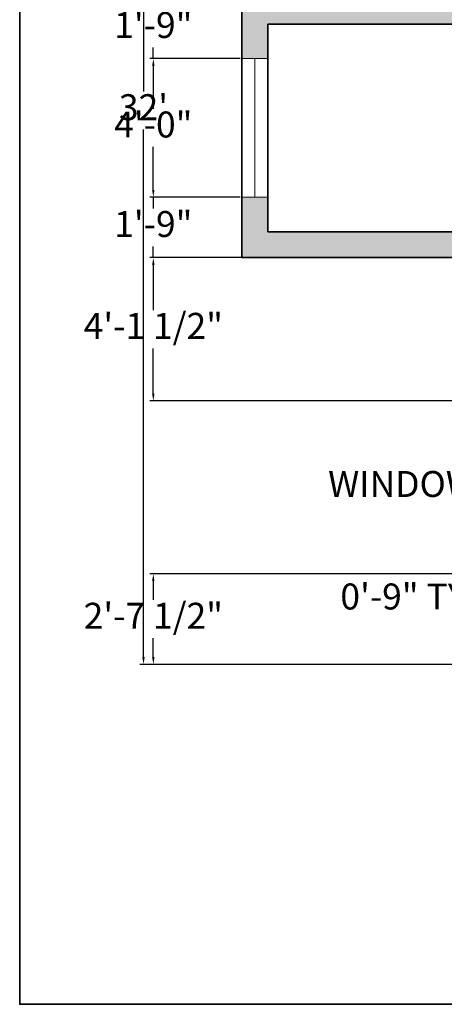
# Model space of a CAD drawing. Units: inches. Extents: x 1329 to 1989, y 1493 to 2072.
# Tile 1 of 4: x 1329 to 1476, y 1501 to 1842. Entities that reach past the tile are written whole.
import ezdxf

# ---------------------------------------------------------------- set-up
doc = ezdxf.new("R2010")
doc.units = ezdxf.units.IN
for name, color, linetype, lineweight in [('A-ANNO-DIMS', 2, 'Continuous', 18), ('A-ANNO-TTLB', 7, 'Continuous', 35), ('A-GLAZ', 4, 'Continuous', 18), ('A-WALL', 7, 'Continuous', 35)]:
    doc.layers.add(name, color=color, linetype=linetype, lineweight=lineweight)
doc.layers.add('A-WALL-PATT', color=251, linetype='Continuous', lineweight=13, true_color=0x636466)
doc.styles.get("Standard").update_dxf_attribs({"font": 'arial.ttf'})
doc.dimstyles.new('ISO-25', dxfattribs={"dimtxt": 9, "dimasz": 2.5, "dimexe": 1.25, "dimexo": 0.625, "dimgap": 2, "dimtad": 0, "dimtih": 1, "dimtoh": 1, "dimdec": 1, "dimlunit": 4, "dimtxsty": 'Standard', "dimcen": 2.5, "dimadec": 0, "dimazin": 0, "dimtfac": 0.5, "dimtdec": 1, "dimtmove": 0, "dimatfit": 3, "dimfxl": 1, "dimarcsym": 0})

# ---------------------------------------------------------------- blocks, each defined once
blk = doc.blocks.new('*D14')
at = {"layer": 'A-ANNO-DIMS', "color": 0, "lineweight": -2, "transparency": 16777216}
for p, q in [((1499.06, 2002.52), (1370.79, 2002.52)), ((1372.04, 2000.02), (1372.04, 1817.12)), ((1372.04, 1621.02), (1372.04, 1803.93)), ((1499.06, 1618.52), (1370.79, 1618.52))]:
    blk.add_line(p, q, dxfattribs=at)
at = {"layer": 'A-ANNO-DIMS', "color": 0, "transparency": 16777216}
for points in [[(1371.62, 2000.02), (1372.45, 2000.02), (1372.04, 2002.52)], [(1371.62, 1621.02), (1372.45, 1621.02), (1372.04, 1618.52)]]:
    blk.add_solid(points, dxfattribs=at)
at = {"layer": 'Defpoints', "color": 0, "transparency": 16777216}
for p in [(1499.69, 2002.52), (1372.04, 1618.52), (1499.69, 1618.52)]:
    blk.add_point(p, dxfattribs=at)
at = {"layer": 'A-ANNO-DIMS', "color": 0, "transparency": 16777216, "insert": (1372.04, 1810.52), "char_height": 9, "attachment_point": 5}
blk.add_mtext("32'", dxfattribs=at)
blk = doc.blocks.new('*D17')
at = {"layer": 'A-ANNO-DIMS', "color": 0, "lineweight": -2, "transparency": 16777216}
for p, q in [((1499.06, 1709.88), (1489.44, 1709.88)), ((1490.69, 1707.38), (1490.69, 1686.53)), ((1490.69, 1652.38), (1490.69, 1673.22)), ((1499.06, 1649.88), (1489.44, 1649.88))]:
    blk.add_line(p, q, dxfattribs=at)
at = {"layer": 'A-ANNO-DIMS', "color": 0, "transparency": 16777216}
for points in [[(1490.27, 1707.38), (1491.1, 1707.38), (1490.69, 1709.88)], [(1490.27, 1652.38), (1491.1, 1652.38), (1490.69, 1649.88)]]:
    blk.add_solid(points, dxfattribs=at)
at = {"layer": 'Defpoints', "color": 0, "transparency": 16777216}
for p in [(1490.69, 1709.88), (1499.69, 1709.88), (1499.69, 1649.88)]:
    blk.add_point(p, dxfattribs=at)
at = {"layer": 'A-ANNO-DIMS', "color": 0, "transparency": 16777216, "insert": (1490.69, 1679.88), "char_height": 9, "attachment_point": 5}
blk.add_mtext('WINDOW 5\'-0" TYP.', dxfattribs=at)
blk = doc.blocks.new('*D18')
at = {"layer": 'A-ANNO-DIMS', "color": 0, "lineweight": -2, "transparency": 16777216}
for p, q in [((1499.69, 1649.25), (1499.69, 1639.63)), ((1508.69, 1649.25), (1508.69, 1639.63)), ((1499.69, 1640.88), (1497.19, 1640.88)), ((1506.19, 1640.88), (1502.19, 1640.88))]:
    blk.add_line(p, q, dxfattribs=at)
at = {"layer": 'A-ANNO-DIMS', "color": 0, "transparency": 16777216}
for points in [[(1502.19, 1641.29), (1502.19, 1640.46), (1499.69, 1640.88)], [(1506.19, 1641.29), (1506.19, 1640.46), (1508.69, 1640.88)]]:
    blk.add_solid(points, dxfattribs=at)
at = {"layer": 'Defpoints', "color": 0, "transparency": 16777216}
for p in [(1499.69, 1649.88), (1508.69, 1649.88), (1499.69, 1640.88)]:
    blk.add_point(p, dxfattribs=at)
at = {"layer": 'A-ANNO-DIMS', "color": 0, "transparency": 16777216, "insert": (1467.76, 1640.88), "char_height": 9, "attachment_point": 5}
blk.add_mtext('0\'-9" TYP.', dxfattribs=at)
blk = doc.blocks.new('*D46')
at = {"layer": 'A-ANNO-DIMS', "color": 0, "lineweight": -2, "transparency": 16777216}
for p, q in [((1405.52, 1828.52), (1374.19, 1828.52)), ((1375.44, 1826.02), (1375.44, 1811.12)), ((1375.44, 1783.02), (1375.44, 1797.93)), ((1405.52, 1780.52), (1374.19, 1780.52))]:
    blk.add_line(p, q, dxfattribs=at)
at = {"layer": 'A-ANNO-DIMS', "color": 0, "transparency": 16777216}
for points in [[(1375.02, 1826.02), (1375.86, 1826.02), (1375.44, 1828.52)], [(1375.02, 1783.02), (1375.86, 1783.02), (1375.44, 1780.52)]]:
    blk.add_solid(points, dxfattribs=at)
at = {"layer": 'Defpoints', "color": 0, "transparency": 16777216}
for p in [(1406.14, 1828.52), (1375.44, 1780.52), (1406.14, 1780.52)]:
    blk.add_point(p, dxfattribs=at)
at = {"layer": 'A-ANNO-DIMS', "color": 0, "transparency": 16777216, "insert": (1375.44, 1804.52), "char_height": 9, "attachment_point": 5}
blk.add_mtext('4\'-0"', dxfattribs=at)
blk = doc.blocks.new('*D47')
at = {"layer": 'A-ANNO-DIMS', "color": 0, "lineweight": -2, "transparency": 16777216}
for p, q in [((1375.44, 1852.02), (1375.44, 1854.52)), ((1405.52, 1849.52), (1374.19, 1849.52)), ((1375.44, 1849.52), (1375.44, 1845.62)), ((1375.44, 1828.52), (1375.44, 1832.43)), ((1405.52, 1828.52), (1374.19, 1828.52)), ((1375.44, 1826.02), (1375.44, 1823.52))]:
    blk.add_line(p, q, dxfattribs=at)
at = {"layer": 'A-ANNO-DIMS', "color": 0, "transparency": 16777216}
for points in [[(1375.02, 1852.02), (1375.86, 1852.02), (1375.44, 1849.52)], [(1375.02, 1826.02), (1375.86, 1826.02), (1375.44, 1828.52)]]:
    blk.add_solid(points, dxfattribs=at)
at = {"layer": 'Defpoints', "color": 0, "transparency": 16777216}
for p in [(1406.14, 1849.52), (1375.44, 1828.52), (1406.14, 1828.52)]:
    blk.add_point(p, dxfattribs=at)
at = {"layer": 'A-ANNO-DIMS', "color": 0, "transparency": 16777216, "insert": (1375.44, 1839.02), "char_height": 9, "attachment_point": 5}
blk.add_mtext('1\'-9"', dxfattribs=at)
blk = doc.blocks.new('*D48')
at = {"layer": 'A-ANNO-DIMS', "color": 0, "lineweight": -2, "transparency": 16777216}
for p, q in [((1375.44, 1783.02), (1375.44, 1785.52)), ((1405.52, 1780.52), (1374.19, 1780.52)), ((1375.44, 1780.52), (1375.44, 1776.62)), ((1375.44, 1759.52), (1375.44, 1763.43)), ((1405.52, 1759.52), (1374.19, 1759.52)), ((1375.44, 1757.02), (1375.44, 1754.52))]:
    blk.add_line(p, q, dxfattribs=at)
at = {"layer": 'A-ANNO-DIMS', "color": 0, "transparency": 16777216}
for points in [[(1375.02, 1783.02), (1375.86, 1783.02), (1375.44, 1780.52)], [(1375.02, 1757.02), (1375.86, 1757.02), (1375.44, 1759.52)]]:
    blk.add_solid(points, dxfattribs=at)
at = {"layer": 'Defpoints', "color": 0, "transparency": 16777216}
for p in [(1406.14, 1780.52), (1375.44, 1759.52), (1406.14, 1759.52)]:
    blk.add_point(p, dxfattribs=at)
at = {"layer": 'A-ANNO-DIMS', "color": 0, "transparency": 16777216, "insert": (1375.44, 1770.02), "char_height": 9, "attachment_point": 5}
blk.add_mtext('1\'-9"', dxfattribs=at)
blk = doc.blocks.new('*D49')
at = {"layer": 'A-ANNO-DIMS', "color": 0, "lineweight": -2, "transparency": 16777216}
for p, q in [((1499.06, 1759.52), (1374.19, 1759.52)), ((1375.44, 1757.02), (1375.44, 1741.35)), ((1375.44, 1712.38), (1375.44, 1728.05)), ((1499.06, 1709.88), (1374.19, 1709.88))]:
    blk.add_line(p, q, dxfattribs=at)
at = {"layer": 'A-ANNO-DIMS', "color": 0, "transparency": 16777216}
for points in [[(1375.02, 1757.02), (1375.86, 1757.02), (1375.44, 1759.52)], [(1375.02, 1712.38), (1375.86, 1712.38), (1375.44, 1709.88)]]:
    blk.add_solid(points, dxfattribs=at)
at = {"layer": 'Defpoints', "color": 0, "transparency": 16777216}
for p in [(1375.44, 1759.52), (1499.69, 1759.52), (1499.69, 1709.88)]:
    blk.add_point(p, dxfattribs=at)
at = {"layer": 'A-ANNO-DIMS', "color": 0, "transparency": 16777216, "insert": (1375.44, 1734.7), "char_height": 9, "attachment_point": 5}
blk.add_mtext('4\'-1 1/2"', dxfattribs=at)
blk = doc.blocks.new('*D50')
at = {"layer": 'A-ANNO-DIMS', "color": 0, "lineweight": -2, "transparency": 16777216}
for p, q in [((1499.06, 1649.88), (1374.19, 1649.88)), ((1375.44, 1647.38), (1375.44, 1640.85)), ((1375.44, 1621.02), (1375.44, 1627.55)), ((1499.06, 1618.52), (1374.19, 1618.52))]:
    blk.add_line(p, q, dxfattribs=at)
at = {"layer": 'A-ANNO-DIMS', "color": 0, "transparency": 16777216}
for points in [[(1375.02, 1647.38), (1375.86, 1647.38), (1375.44, 1649.88)], [(1375.02, 1621.02), (1375.86, 1621.02), (1375.44, 1618.52)]]:
    blk.add_solid(points, dxfattribs=at)
at = {"layer": 'Defpoints', "color": 0, "transparency": 16777216}
for p in [(1499.69, 1649.88), (1375.44, 1618.52), (1499.69, 1618.52)]:
    blk.add_point(p, dxfattribs=at)
at = {"layer": 'A-ANNO-DIMS', "color": 0, "transparency": 16777216, "insert": (1375.44, 1634.2), "char_height": 9, "attachment_point": 5}
blk.add_mtext('2\'-7 1/2"', dxfattribs=at)

msp = doc.modelspace()

# ---------------------------------------------------------------- hatches: boundary and pattern name
at = {"layer": 'A-WALL-PATT'}
h = msp.add_hatch(color=256, dxfattribs=at)
h.dxf.hatch_style = 1
h.paths.add_polyline_path([(1550.69, 2002.52), (1499.69, 2002.52), (1499.69, 1951.52), (1508.69, 1951.52), (1508.69, 1993.52), (1550.69, 1993.52)])
h.paths.add_polyline_path([(1670.69, 2002.52), (1610.69, 2002.52), (1610.69, 1993.52), (1652.69, 1993.52), (1652.69, 1885.52), (1658.69, 1885.52), (1658.69, 1903.52), (1706.69, 1903.52), (1712.69, 1903.52), (1712.69, 1909.52), (1706.69, 1909.52), (1658.69, 1909.52), (1658.69, 1993.52), (1670.69, 1993.52)])
h.paths.add_polyline_path([(1721.69, 2002.52), (1694.69, 2002.52), (1694.69, 1993.52), (1706.69, 1993.52), (1706.69, 1939.52), (1712.69, 1939.52), (1730.69, 1939.52), (1730.69, 1945.52), (1712.69, 1945.52), (1712.69, 1993.52), (1721.69, 1993.52)])
h.paths.add_polyline_path([(1790.69, 2002.52), (1745.69, 2002.52), (1745.69, 1993.52), (1754.69, 1993.52), (1754.69, 1945.52), (1754.69, 1939.52), (1754.69, 1885.52), (1760.69, 1885.52), (1760.69, 1993.52), (1790.69, 1993.52)])
h.paths.add_polyline_path([(1889.69, 2002.52), (1850.69, 2002.52), (1850.69, 1993.52), (1880.69, 1993.52), (1880.69, 1951.52), (1889.69, 1951.52)])
h.paths.add_polyline_path([(1889.69, 1891.52), (1880.69, 1891.52), (1880.69, 1849.52), (1760.69, 1849.52), (1754.69, 1849.52), (1688.69, 1849.52), (1688.69, 1843.52), (1697.69, 1843.52), (1760.69, 1843.52), (1880.69, 1843.52), (1880.69, 1798.52), (1889.69, 1798.52)])
h.paths.add_polyline_path([(1658.69, 1849.52), (1652.69, 1849.52), (1508.69, 1849.52), (1508.69, 1891.52), (1499.69, 1891.52), (1499.69, 1849.52), (1406.14, 1849.52), (1406.14, 1828.52), (1415.14, 1828.52), (1415.14, 1840.52), (1508.69, 1840.52), (1652.69, 1840.52), (1658.69, 1840.52)])
h.paths.add_polyline_path([(1658.69, 1804.52), (1652.69, 1804.52), (1652.69, 1768.52), (1508.69, 1768.52), (1415.14, 1768.52), (1415.14, 1780.52), (1406.14, 1780.52), (1406.14, 1759.52), (1499.69, 1759.52), (1499.69, 1709.88), (1508.69, 1709.88), (1508.69, 1759.52), (1658.69, 1759.52)])
h.paths.add_polyline_path([(1508.69, 1649.88), (1499.69, 1649.88), (1499.69, 1618.52), (1568.69, 1618.52), (1568.69, 1627.52), (1508.69, 1627.52)])
h.paths.add_polyline_path([(1697.69, 1684.52), (1697.69, 1693.52), (1697.69, 1795.52), (1688.69, 1795.52), (1688.69, 1693.52), (1688.69, 1684.52), (1688.69, 1627.52), (1628.69, 1627.52), (1628.69, 1618.52), (1688.69, 1618.52), (1688.69, 1588.52), (1697.69, 1588.52), (1697.69, 1618.52)])
h.paths.add_polyline_path([(1790.69, 1693.52), (1760.69, 1693.52), (1745.69, 1693.52), (1745.69, 1684.52), (1760.69, 1684.52), (1790.69, 1684.52)])
h.paths.add_polyline_path([(1889.69, 1738.52), (1880.69, 1738.52), (1880.69, 1693.52), (1850.69, 1693.52), (1850.69, 1684.52), (1880.69, 1684.52), (1889.69, 1684.52)])

# ---------------------------------------------------------------- linework, layer by layer
at = {"layer": 'A-ANNO-TTLB'}
msp.add_lwpolyline([(1329.11, 2071.84), (1964.17, 2071.84), (1964.17, 1500.65), (1329.11, 1500.65)], close=True, dxfattribs=at)
at = {"layer": 'A-GLAZ'}
for p, q in [((1415.14, 1828.52), (1406.14, 1828.52)), ((1410.64, 1828.52), (1410.64, 1780.52)), ((1415.14, 1780.52), (1406.14, 1780.52))]:
    msp.add_line(p, q, dxfattribs=at)
at = {"layer": 'A-WALL'}
for p, q in [((1406.14, 1759.52), (1406.14, 1849.52)), ((1508.69, 1840.52), (1415.14, 1840.52)), ((1415.14, 1768.52), (1415.14, 1840.52)), ((1508.69, 1768.52), (1415.14, 1768.52)), ((1499.69, 1759.52), (1406.14, 1759.52))]:
    msp.add_line(p, q, dxfattribs=at)

# ---------------------------------------------------------------- dimensions: what is measured, and where the dimension line sits
at = {"layer": 'A-ANNO-DIMS'}
for base, p1, p2, override, picture, middle in [((1372.04, 1618.52), (1499.69, 2002.52), (1499.69, 1618.52), {"dimclrd": 0, "dimclre": 0, "dimclrt": 0}, '*D14', (1372.04, 1810.52)), ((1375.44, 1828.52), (1406.14, 1849.52), (1406.14, 1828.52), {"dimdec": 1, "dimlfac": 1, "dimrnd": 0, "dimzin": 1, "dimdsep": 46, "dimlunit": 4, "dimfrac": 2}, '*D47', (1375.44, 1839.02)), ((1375.44, 1780.52), (1406.14, 1828.52), (1406.14, 1780.52), {"dimdec": 1, "dimlfac": 1, "dimrnd": 0, "dimzin": 1, "dimdsep": 46, "dimlunit": 4, "dimfrac": 2}, '*D46', (1375.44, 1804.52)), ((1375.44, 1759.52), (1406.14, 1780.52), (1406.14, 1759.52), {"dimdec": 1, "dimlfac": 1, "dimrnd": 0, "dimzin": 1, "dimdsep": 46, "dimlunit": 4, "dimfrac": 2}, '*D48', (1375.44, 1770.02)), ((1375.44, 1759.52), (1499.69, 1709.88), (1499.69, 1759.52), {"dimdec": 1, "dimlfac": 1, "dimrnd": 0, "dimzin": 1, "dimdsep": 46, "dimlunit": 4, "dimfrac": 2}, '*D49', (1375.44, 1734.7)), ((1375.44, 1618.52), (1499.69, 1649.88), (1499.69, 1618.52), {"dimdec": 1, "dimlfac": 1, "dimrnd": 0, "dimzin": 1, "dimdsep": 46, "dimlunit": 4, "dimfrac": 2}, '*D50', (1375.44, 1634.2))]:
    dim = msp.add_linear_dim(base=base, p1=p1, p2=p2, angle=90, dimstyle='ISO-25', override=override, dxfattribs=at)
    dim.commit()
    dim.dimension.update_dxf_attribs({"geometry": picture, "text_midpoint": middle})
for base, p1, p2, angle, text, picture, middle in [((1490.69, 1709.88), (1499.69, 1649.88), (1499.69, 1709.88), 90, 'WINDOW <> TYP.', '*D17', (1490.69, 1679.88)), ((1499.69, 1640.88), (1508.69, 1649.88), (1499.69, 1649.88), 180, '<> TYP.', '*D18', (1467.76, 1640.88))]:
    dim = msp.add_linear_dim(base=base, p1=p1, p2=p2, angle=angle, text=text, dimstyle='ISO-25', override={"dimdec": 1, "dimlfac": 1, "dimrnd": 0, "dimzin": 1, "dimdsep": 46, "dimlunit": 4, "dimfrac": 2}, dxfattribs=at)
    dim.commit()
    dim.dimension.update_dxf_attribs({"geometry": picture, "text_midpoint": middle})

doc.saveas('drawing.dxf')
